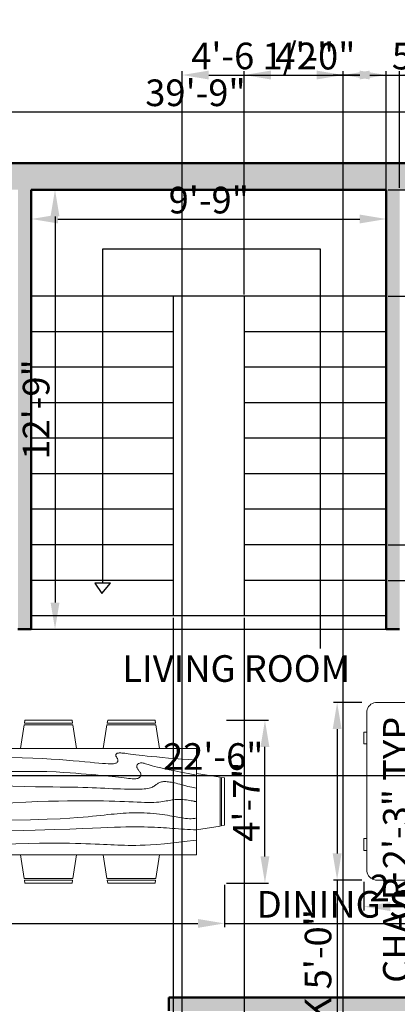
# Model space of a CAD drawing. Units: inches. Extents: x 875413 to 876020, y 447446 to 448210.
# Tile 6 of 8: x 875639 to 875767, y 447795 to 448127. Entities that reach past the tile are written whole.
import ezdxf

# ---------------------------------------------------------------- set-up
doc = ezdxf.new("R2010")
doc.units = ezdxf.units.IN
for name, color, linetype, lineweight in [('A-ANNO-DIMS', 2, 'Continuous', 13), ('A-AREA-IDEN', 7, 'Continuous', 25), ('A-FLOR-STRS', 7, 'Continuous', 25), ('A-FURN', 8, 'Continuous', 18), ('A-WALL', 7, 'Continuous', 50)]:
    doc.layers.add(name, color=color, linetype=linetype, lineweight=lineweight)
doc.layers.add('A-WALL-PATT', color=18, linetype='Continuous', lineweight=13, true_color=0x000000)
doc.styles.get("Standard").update_dxf_attribs({"font": 'arial.ttf'})
doc.dimstyles.new('ISO-25', dxfattribs={"dimtxt": 9, "dimasz": 9, "dimexe": 1.25, "dimexo": 0.625, "dimtad": 1, "dimdec": 1, "dimrnd": 9, "dimlunit": 3, "dimtxsty": 'Standard', "dimcen": 2.5, "dimadec": 0, "dimazin": 0, "dimtfac": 1, "dimtdec": 1, "dimtmove": 0, "dimatfit": 3, "dimfxl": 1, "dimarcsym": 0})

# ---------------------------------------------------------------- blocks, each defined once
blk = doc.blocks.new('*D3')
at = {"layer": 'A-ANNO-DIMS', "color": 0, "lineweight": -2, "transparency": 16777216}
for p, q in [((875643.2, 448069.39), (875643.2, 448058.87)), ((875763.2, 448069.39), (875763.2, 448058.87)), ((875652.2, 448060.12), (875754.2, 448060.12))]:
    blk.add_line(p, q, dxfattribs=at)
at = {"layer": 'A-ANNO-DIMS', "color": 0, "transparency": 16777216}
for points in [[(875652.2, 448061.62), (875652.2, 448058.62), (875643.2, 448060.12)], [(875754.2, 448061.62), (875754.2, 448058.62), (875763.2, 448060.12)]]:
    blk.add_solid(points, dxfattribs=at)
at = {"layer": 'Defpoints', "color": 0, "transparency": 16777216}
for p in [(875643.2, 448070.02), (875763.2, 448070.02), (875763.2, 448060.12)]:
    blk.add_point(p, dxfattribs=at)
at = {"layer": 'A-ANNO-DIMS', "color": 0, "transparency": 16777216, "insert": (875703.2, 448065.34), "char_height": 9, "attachment_point": 5}
blk.add_mtext('9\'-9"', dxfattribs=at)
blk = doc.blocks.new('*D4')
at = {"layer": 'A-ANNO-DIMS', "color": 0, "lineweight": -2, "transparency": 16777216}
for p, q in [((875643.83, 448070.02), (875652.48, 448070.02)), ((875651.23, 448061.02), (875651.23, 447930.52)), ((875643.83, 447921.52), (875652.48, 447921.52))]:
    blk.add_line(p, q, dxfattribs=at)
at = {"layer": 'A-ANNO-DIMS', "color": 0, "transparency": 16777216}
for points in [[(875649.73, 448061.02), (875652.73, 448061.02), (875651.23, 448070.02)], [(875649.73, 447930.52), (875652.73, 447930.52), (875651.23, 447921.52)]]:
    blk.add_solid(points, dxfattribs=at)
at = {"layer": 'Defpoints', "color": 0, "transparency": 16777216}
for p in [(875643.2, 448070.02), (875643.2, 447921.52), (875651.23, 447921.52)]:
    blk.add_point(p, dxfattribs=at)
at = {"layer": 'A-ANNO-DIMS', "color": 0, "transparency": 16777216, "insert": (875646.01, 447995.77), "char_height": 9, "attachment_point": 5, "rotation": 90}
blk.add_mtext('12\'-9"', dxfattribs=at)
blk = doc.blocks.new('*D13')
at = {"layer": 'A-ANNO-DIMS', "color": 0, "lineweight": -2, "transparency": 16777216}
for p, q in [((875571.2, 447920.89), (875571.2, 447870.86)), ((875838.2, 447920.89), (875838.2, 447870.86)), ((875580.2, 447872.11), (875829.2, 447872.11))]:
    blk.add_line(p, q, dxfattribs=at)
at = {"layer": 'A-ANNO-DIMS', "color": 0, "transparency": 16777216}
for points in [[(875580.2, 447873.61), (875580.2, 447870.61), (875571.2, 447872.11)], [(875829.2, 447873.61), (875829.2, 447870.61), (875838.2, 447872.11)]]:
    blk.add_solid(points, dxfattribs=at)
at = {"layer": 'Defpoints', "color": 0, "transparency": 16777216}
for p in [(875571.2, 447921.52), (875838.2, 447921.52), (875838.2, 447872.11)]:
    blk.add_point(p, dxfattribs=at)
at = {"layer": 'A-ANNO-DIMS', "color": 0, "transparency": 16777216, "insert": (875704.7, 447877.33), "char_height": 9, "attachment_point": 5}
blk.add_mtext('22\'-6"', dxfattribs=at)
blk = doc.blocks.new('Dining Set - 36 x 72 in.')
for p, q in [((-22, 27.5), (-22.1562, 26.50042)), ((-22, 27.5), (-6, 27.5)), ((-5.8437, 26.49966), (-6, 27.5)), ((6, 27.5), (5.8438, 26.50042)), ((6, 27.5), (22, 27.5)), ((22.1563, 26.49966), (22, 27.5)), ((-22.2343, 26.00059), (-23.4847, 17.99762)), ((-22.2304, 26), (-5.7608, 26)), ((-5.8416, 26.5), (-22.1534, 26.5)), ((-4.5152, 17.99762), (-5.7655, 25.99926)), ((5.7657, 26.00059), (4.5153, 17.99762)), ((5.7696, 26), (22.2392, 26)), ((22.1584, 26.5), (5.8466, 26.5)), ((23.4848, 17.99762), (22.2345, 25.99926)), ((36, 18), (-36, 18)), ((-36, 18), (-36, -18)), ((36, -18), (36, 18)), ((-45.5, 8), (-44.5004, 8.15617)), ((-45.5, 8), (-45.5, -8)), ((-44.5, -8.15843), (-44.5, 8.15338)), ((-44.0006, 8.23428), (-35.9976, 9.48474)), ((-44, 8.23041), (-44, -8.23915)), ((44.0006, 8.23428), (35.9976, 9.48474)), ((44, 8.23041), (44, -8.23915)), ((44.5, -8.15843), (44.5, 8.15338)), ((45.5, 8), (44.5005, 8.15617)), ((45.5, 8), (45.5, -8)), ((-44.4997, -8.15631), (-45.5, -8)), ((-35.9976, -9.48476), (-43.9993, -8.2345)), ((35.9976, -9.48476), (43.9993, -8.2345)), ((44.4997, -8.15631), (45.5, -8)), ((-36, -18), (36, -18)), ((-22.2343, -26.0006), (-23.4847, -17.99762)), ((-4.5152, -17.99762), (-5.7655, -25.99928)), ((5.7657, -26.0006), (4.5153, -17.99762)), ((23.4848, -17.99762), (22.2345, -25.99928)), ((-22.2304, -26), (-5.7608, -26)), ((-22, -27.5), (-22.1562, -26.50044)), ((-5.8416, -26.5), (-22.1534, -26.5)), ((-5.8437, -26.49967), (-6, -27.5)), ((5.7696, -26), (22.2392, -26)), ((6, -27.5), (5.8438, -26.50044)), ((22.1584, -26.5), (5.8466, -26.5)), ((22.1563, -26.49967), (22, -27.5)), ((-22, -27.5), (-6, -27.5)), ((6, -27.5), (22, -27.5))]:
    blk.add_line(p, q)
for points in [[(-36, 15), (-31.1772, 14.97754), (-26.8079, 14.91406), (-22.8538, 14.81543), (-19.276, 14.6875), (-16.0362, 14.53613), (-13.0957, 14.36718), (-10.4159, 14.18652), (-7.9583, 14), (-5.6904, 13.81315), (-3.6035, 13.63021), (-1.6954, 13.45508), (0.0365, 13.29166), (1.5945, 13.14388), (2.9811, 13.01562), (4.1988, 12.9108), (5.25, 12.83333), (6.1393, 12.78613), (6.8802, 12.76823), (7.4883, 12.77767), (7.9792, 12.8125), (8.3685, 12.87077), (8.6719, 12.95052), (8.9049, 13.0498), (9.0833, 13.16666), (9.2205, 13.29899), (9.3216, 13.44401), (9.3895, 13.59879), (9.4271, 13.76041), (9.4373, 13.92594), (9.4232, 14.09245), (9.3875, 14.257), (9.3333, 14.41666), (9.2638, 14.56917), (9.1836, 14.71484), (9.0975, 14.85465), (9.0104, 14.98958), (8.9272, 15.1206), (8.8529, 15.2487), (8.7922, 15.37483), (8.75, 15.5), (8.7305, 15.62467), (8.7344, 15.74739), (8.7617, 15.86621), (8.8125, 15.97916), (8.8867, 16.08431), (8.9844, 16.17968), (9.1055, 16.26334), (9.25, 16.33333), (9.4189, 16.38802), (9.6172, 16.42708), (9.8506, 16.45052), (10.125, 16.45833), (10.4463, 16.45052), (10.8203, 16.42708), (11.2529, 16.38802), (11.75, 16.33333), (12.3184, 16.26318), (12.9694, 16.17838), (13.7151, 16.07991), (14.5677, 15.96875), (15.5395, 15.84586), (16.6426, 15.71224), (17.8893, 15.56884), (19.2917, 15.41666), (20.859, 15.25667), (22.5879, 15.08984), (24.4721, 14.91715), (26.5052, 14.73958), (28.6809, 14.5581), (30.9929, 14.3737), (33.4347, 14.18733), (36, 14)], [(-36, 10), (-28.9766, 10.14274), (-23.1725, 10.20442), (-18.4241, 10.19775), (-14.5677, 10.13541), (-11.4399, 10.03011), (-8.877, 9.89453), (-6.7154, 9.74137), (-4.7917, 9.58333), (-2.9698, 9.43082), (-1.2246, 9.28515), (0.4415, 9.14534), (2.026, 9.01041), (3.5266, 8.87939), (4.9408, 8.7513), (6.266, 8.62516), (7.5, 8.5), (8.6411, 8.37549), (9.6914, 8.2539), (10.6538, 8.13818), (11.5312, 8.03125), (12.3267, 7.93603), (13.043, 7.85547), (13.6831, 7.79248), (14.25, 7.75), (14.7471, 7.7303), (15.1797, 7.73307), (15.5537, 7.75732), (15.875, 7.80208), (16.1494, 7.86637), (16.3828, 7.94922), (16.5811, 8.04964), (16.75, 8.16666), (16.8944, 8.29915), (17.0143, 8.44531), (17.1089, 8.60319), (17.1771, 8.77083), (17.218, 8.94629), (17.2305, 9.1276), (17.2137, 9.31282), (17.1667, 9.5), (17.0895, 9.6875), (16.987, 9.875), (16.8649, 10.0625), (16.7292, 10.25), (16.5856, 10.4375), (16.4401, 10.625), (16.2985, 10.8125), (16.1667, 11), (16.05, 11.18733), (15.9518, 11.3737), (15.8752, 11.5581), (15.8229, 11.73958), (15.798, 11.91715), (15.8034, 12.08984), (15.842, 12.25667), (15.9167, 12.41666), (16.0295, 12.56836), (16.1784, 12.70833), (16.3605, 12.83268), (16.5729, 12.9375), (16.8127, 13.01888), (17.0768, 13.07291), (17.3625, 13.0957), (17.6667, 13.08333), (17.9894, 13.03312), (18.3418, 12.94726), (18.7382, 12.82918), (19.1927, 12.68229), (19.7195, 12.51001), (20.3327, 12.31575), (21.0465, 12.10294), (21.875, 11.875), (22.8357, 11.63354), (23.959, 11.37304), (25.2786, 11.08618), (26.8282, 10.76562), (28.6414, 10.40405), (30.752, 9.99414), (33.1936, 9.52856), (36, 9)], [(-36, 5.5), (-30.7157, 5.3348), (-26.069, 5.20963), (-21.9946, 5.11767), (-18.4271, 5.05208), (-15.3009, 5.00602), (-12.5508, 4.97265), (-10.1112, 4.94515), (-7.9167, 4.91666), (-5.909, 4.88167), (-4.0586, 4.83984), (-2.3429, 4.79215), (-0.7396, 4.73958), (0.7739, 4.6831), (2.22, 4.6237), (3.6213, 4.56233), (5, 4.5), (6.373, 4.43782), (7.7344, 4.3776), (9.0723, 4.32129), (10.375, 4.27083), (11.6309, 4.22819), (12.8281, 4.19531), (13.9551, 4.17415), (15, 4.16666), (15.954, 4.17448), (16.819, 4.19791), (17.6001, 4.23698), (18.3021, 4.29166), (18.9299, 4.36198), (19.4883, 4.44791), (19.9823, 4.54948), (20.4167, 4.66666), (20.7969, 4.79899), (21.1302, 4.94401), (21.4245, 5.09879), (21.6875, 5.26041), (21.9271, 5.42594), (22.1511, 5.59245), (22.3672, 5.757), (22.5834, 5.91666), (22.8065, 6.06868), (23.0404, 6.21093), (23.2879, 6.34147), (23.5521, 6.45833), (23.8358, 6.55957), (24.142, 6.64323), (24.4735, 6.70735), (24.8334, 6.75), (25.2235, 6.76969), (25.642, 6.76692), (26.0858, 6.74267), (26.5521, 6.69791), (27.0379, 6.63362), (27.5404, 6.55078), (28.0565, 6.45036), (28.5834, 6.33333), (29.1242, 6.19987), (29.7071, 6.04687), (30.3661, 5.87044), (31.1354, 5.66666), (32.0493, 5.43164), (33.142, 5.16146), (34.4475, 4.85221), (36, 4.5)], [(-36, -1), (-30.7915, -0.6591), (-26.0195, -0.38216), (-21.6519, -0.16284), (-17.6563, 0.00521), (-14.0005, 0.12833), (-10.6523, 0.21289), (-7.5796, 0.26522), (-4.75, 0.29166), (-2.134, 0.29793), (0.2878, 0.28711), (2.5317, 0.26163), (4.6146, 0.22396), (6.5529, 0.17651), (8.3633, 0.12174), (10.0623, 0.06209), (11.6667, 0), (13.1899, -0.06201), (14.6341, -0.1211), (15.9982, -0.17432), (17.2813, -0.21875), (18.4823, -0.25147), (19.6003, -0.26953), (20.6343, -0.27002), (21.5834, -0.25), (22.4481, -0.20768), (23.2357, -0.14584), (23.9549, -0.06836), (24.6146, 0.02083), (25.2235, 0.11784), (25.7904, 0.21875), (26.3241, 0.31966), (26.8334, 0.41666), (27.3265, 0.50618), (27.8099, 0.58593), (28.2894, 0.65397), (28.7709, 0.70833), (29.2601, 0.74707), (29.763, 0.76823), (30.2855, 0.76985), (30.8334, 0.75), (31.4088, 0.70784), (31.9994, 0.64713), (32.589, 0.57275), (33.1615, 0.48958), (33.7008, 0.4025), (34.1908, 0.3164), (34.6153, 0.23616), (34.9584, 0.16666), (35.2099, 0.11165), (35.3848, 0.07031), (35.504, 0.04069), (35.5886, 0.02083), (35.6594, 0.00879), (35.7377, 0.0026), (35.8442, 0.00032), (36, 0)], [(-36, -6.5), (-27.1843, -6.31267), (-20.084, -6.1263), (-14.469, -5.9419), (-10.1094, -5.76042), (-6.7752, -5.58285), (-4.2363, -5.41016), (-2.2629, -5.24333), (-0.625, -5.08334), (0.8708, -4.93099), (2.2715, -4.78646), (3.5872, -4.64974), (4.8281, -4.52084), (6.0046, -4.39974), (7.127, -4.28646), (8.2053, -4.18099), (9.25, -4.08334), (10.2705, -3.99382), (11.2734, -3.91407), (12.2647, -3.84603), (13.25, -3.79167), (14.2354, -3.75293), (15.2266, -3.73177), (16.2295, -3.73015), (17.25, -3.75), (18.2912, -3.79248), (19.3451, -3.85547), (20.4009, -3.93604), (21.4479, -4.03125), (22.4754, -4.13819), (23.4727, -4.25391), (24.4289, -4.37549), (25.3334, -4.5), (26.1785, -4.62492), (26.9694, -4.74935), (27.7145, -4.87281), (28.4219, -4.99479), (29.1, -5.11483), (29.7572, -5.23242), (30.4016, -5.34709), (31.0417, -5.45834), (31.6837, -5.56437), (32.3262, -5.65821), (32.9658, -5.73153), (33.599, -5.77604), (34.2224, -5.78345), (34.8327, -5.74545), (35.4264, -5.65373), (36, -5.5)], [(-36, -10), (-26.4022, -9.81299), (-18.4675, -9.62891), (-11.9839, -9.45069), (-6.7396, -9.28125), (-2.5226, -9.12354), (0.8789, -8.98047), (3.6769, -8.85498), (6.0833, -8.75), (8.2767, -8.66765), (10.3021, -8.60677), (12.1712, -8.56543), (13.8958, -8.54167), (15.4876, -8.53353), (16.9583, -8.53907), (18.3197, -8.55632), (19.5834, -8.58334), (20.7616, -8.61841), (21.8685, -8.66081), (22.9188, -8.71004), (23.9271, -8.76563), (24.9081, -8.82707), (25.8763, -8.89388), (26.8465, -8.96558), (27.8334, -9.04167), (28.8474, -9.12118), (29.8828, -9.20117), (30.93, -9.27824), (31.9792, -9.34896), (33.0205, -9.40991), (34.0443, -9.45768), (35.0407, -9.48885), (36, -9.5)], [(-36, -14.5), (-30.0881, -14.33513), (-25.0332, -14.21224), (-20.7312, -14.12647), (-17.0781, -14.07292), (-13.97, -14.04671), (-11.3027, -14.04297), (-8.9724, -14.05681), (-6.875, -14.08334), (-4.9224, -14.11833), (-3.0905, -14.16016), (-1.3709, -14.20785), (0.2448, -14.26042), (1.7647, -14.3169), (3.1973, -14.3763), (4.5507, -14.43767), (5.8333, -14.5), (7.0554, -14.5621), (8.235, -14.62175), (9.3922, -14.67652), (10.5469, -14.72396), (11.7192, -14.76164), (12.929, -14.78711), (14.1965, -14.79794), (15.5417, -14.79167), (16.9933, -14.76424), (18.6152, -14.70508), (20.4804, -14.60197), (22.6615, -14.44271), (25.2312, -14.21509), (28.2624, -13.9069), (31.8277, -13.50594), (36, -13)]]:
    blk.add_lwpolyline(points)
blk = doc.blocks.new('Desk - 30 x 60 in.')
for p, q in [((-26.999995, 0), (26.999995, 0)), ((-29.999995, -27), (-29.999995, -3)), ((29.999995, -3), (29.999995, -27)), ((26.999995, -30), (-26.999995, -30)), ((-20.000005, -30), (-20.000005, -31)), ((-20.000005, -31), (-16.000005, -31)), ((-16.000005, -31), (-16.000005, -30)), ((15.999995, -31), (15.999995, -30)), ((19.999995, -31), (15.999995, -31)), ((19.999995, -30), (19.999995, -31))]:
    blk.add_line(p, q)
for centre, start, end in [((-26.499995, -3.5), 98.1301, 171.8699), ((26.499995, -3.5), 8.130102, 81.8699), ((-26.499995, -26.5), 188.1301, 261.8699), ((26.499995, -26.5), 278.1301, 351.8699)]:
    blk.add_arc(centre, 3.535534, start, end)
blk = doc.blocks.new('*D37')
at = {"layer": 'A-ANNO-DIMS', "color": 0, "lineweight": -2, "transparency": 16777216}
for p, q in [((875461.7, 448079.64), (875461.7, 448097.63)), ((875470.7, 448096.38), (875926.7, 448096.38)), ((875935.7, 448079.64), (875935.7, 448097.63))]:
    blk.add_line(p, q, dxfattribs=at)
at = {"layer": 'A-ANNO-DIMS', "color": 0, "transparency": 16777216}
for points in [[(875470.7, 448097.88), (875470.7, 448094.88), (875461.7, 448096.38)], [(875926.7, 448097.88), (875926.7, 448094.88), (875935.7, 448096.38)]]:
    blk.add_solid(points, dxfattribs=at)
at = {"layer": 'Defpoints', "color": 0, "transparency": 16777216}
for p in [(875935.7, 448096.38), (875461.7, 448079.02), (875935.7, 448079.02)]:
    blk.add_point(p, dxfattribs=at)
at = {"layer": 'A-ANNO-DIMS', "color": 0, "transparency": 16777216, "insert": (875698.7, 448101.6), "char_height": 9, "attachment_point": 5}
blk.add_mtext('39\'-9"', dxfattribs=at)
blk = doc.blocks.new('*D53')
at = {"layer": 'A-ANNO-DIMS', "color": 0, "lineweight": -2, "transparency": 16777216}
for p, q in [((875617.53, 447835.12), (875617.53, 447820.85)), ((875708.53, 447835.12), (875708.53, 447820.85)), ((875626.53, 447822.1), (875699.53, 447822.1)), ((875708.53, 447822.1), (875817.7, 447822.1))]:
    blk.add_line(p, q, dxfattribs=at)
at = {"layer": 'A-ANNO-DIMS', "color": 0, "transparency": 16777216}
for points in [[(875626.53, 447823.6), (875626.53, 447820.6), (875617.53, 447822.1)], [(875699.53, 447823.6), (875699.53, 447820.6), (875708.53, 447822.1)]]:
    blk.add_solid(points, dxfattribs=at)
at = {"layer": 'Defpoints', "color": 0, "transparency": 16777216}
for p in [(875617.53, 447835.75), (875708.53, 447835.75), (875708.53, 447822.1)]:
    blk.add_point(p, dxfattribs=at)
at = {"layer": 'A-ANNO-DIMS', "color": 0, "transparency": 16777216, "insert": (875767.62, 447827.38), "char_height": 9, "attachment_point": 5}
blk.add_mtext('DINING SET 7\'-7"', dxfattribs=at)
blk = doc.blocks.new('*D54')
at = {"layer": 'A-ANNO-DIMS', "color": 0, "lineweight": -2, "transparency": 16777216}
for p, q in [((875709.16, 447890.75), (875723.43, 447890.75)), ((875722.18, 447844.75), (875722.18, 447881.75)), ((875709.16, 447835.75), (875723.43, 447835.75))]:
    blk.add_line(p, q, dxfattribs=at)
at = {"layer": 'A-ANNO-DIMS', "color": 0, "transparency": 16777216}
for points in [[(875720.68, 447881.75), (875723.68, 447881.75), (875722.18, 447890.75)], [(875720.68, 447844.75), (875723.68, 447844.75), (875722.18, 447835.75)]]:
    blk.add_solid(points, dxfattribs=at)
at = {"layer": 'Defpoints', "color": 0, "transparency": 16777216}
for p in [(875708.53, 447890.75), (875722.18, 447890.75), (875708.53, 447835.75)]:
    blk.add_point(p, dxfattribs=at)
at = {"layer": 'A-ANNO-DIMS', "color": 0, "transparency": 16777216, "insert": (875717.06, 447863.25), "char_height": 9, "attachment_point": 5, "rotation": 90}
blk.add_mtext('4\'-7"', dxfattribs=at)
blk = doc.blocks.new('*D57')
at = {"layer": 'A-ANNO-DIMS', "color": 0, "lineweight": -2, "transparency": 16777216}
for p, q in [((875773.04, 447790.36), (875773.04, 447897.98)), ((875776.46, 447790.36), (875771.79, 447790.36)), ((875773.04, 447772.36), (875773.04, 447781.36)), ((875776.46, 447763.36), (875771.79, 447763.36))]:
    blk.add_line(p, q, dxfattribs=at)
at = {"layer": 'A-ANNO-DIMS', "color": 0, "transparency": 16777216}
for points in [[(875771.54, 447781.36), (875774.54, 447781.36), (875773.04, 447790.36)], [(875771.54, 447772.36), (875774.54, 447772.36), (875773.04, 447763.36)]]:
    blk.add_solid(points, dxfattribs=at)
at = {"layer": 'Defpoints', "color": 0, "transparency": 16777216}
for p in [(875773.04, 447790.36), (875777.09, 447790.36), (875777.09, 447763.36)]:
    blk.add_point(p, dxfattribs=at)
at = {"layer": 'A-ANNO-DIMS', "color": 0, "transparency": 16777216, "insert": (875767.76, 447848.67), "char_height": 9, "attachment_point": 5, "rotation": 90}
blk.add_mtext('CHAIR 2\'-3" TYP.', dxfattribs=at)
blk = doc.blocks.new('*D61')
at = {"layer": 'A-ANNO-DIMS', "color": 0, "lineweight": -2, "transparency": 16777216}
for p, q in [((875754.96, 447896.77), (875745.33, 447896.77)), ((875746.58, 447887.77), (875746.58, 447845.77)), ((875754.96, 447836.77), (875745.33, 447836.77)), ((875746.58, 447836.77), (875746.58, 447765.31))]:
    blk.add_line(p, q, dxfattribs=at)
at = {"layer": 'A-ANNO-DIMS', "color": 0, "transparency": 16777216}
for points in [[(875745.08, 447887.77), (875748.08, 447887.77), (875746.58, 447896.77)], [(875745.08, 447845.77), (875748.08, 447845.77), (875746.58, 447836.77)]]:
    blk.add_solid(points, dxfattribs=at)
at = {"layer": 'Defpoints', "color": 0, "transparency": 16777216}
for p in [(875755.58, 447896.77), (875746.58, 447836.77), (875755.58, 447836.77)]:
    blk.add_point(p, dxfattribs=at)
at = {"layer": 'A-ANNO-DIMS', "color": 0, "transparency": 16777216, "insert": (875741.3, 447796.54), "char_height": 9, "attachment_point": 5, "rotation": 90}
blk.add_mtext('DESK 5\'-0"', dxfattribs=at)
blk = doc.blocks.new('*D62')
at = {"layer": 'A-ANNO-DIMS', "color": 0, "lineweight": -2, "transparency": 16777216}
for p, q in [((875755.58, 447836.14), (875755.58, 447826.52)), ((875786.58, 447836.14), (875786.58, 447826.52)), ((875764.58, 447827.77), (875777.58, 447827.77))]:
    blk.add_line(p, q, dxfattribs=at)
at = {"layer": 'A-ANNO-DIMS', "color": 0, "transparency": 16777216}
for points in [[(875764.58, 447829.27), (875764.58, 447826.27), (875755.58, 447827.77)], [(875777.58, 447829.27), (875777.58, 447826.27), (875786.58, 447827.77)]]:
    blk.add_solid(points, dxfattribs=at)
at = {"layer": 'Defpoints', "color": 0, "transparency": 16777216}
for p in [(875755.58, 447836.77), (875786.58, 447836.77), (875786.58, 447827.77)]:
    blk.add_point(p, dxfattribs=at)
at = {"layer": 'A-ANNO-DIMS', "color": 0, "transparency": 16777216, "insert": (875771.08, 447832.91), "char_height": 9, "attachment_point": 5}
blk.add_mtext('2\'-7"', dxfattribs=at)
blk = doc.blocks.new('*D77')
at = {"layer": 'A-ANNO-DIMS', "color": 0, "lineweight": -2, "transparency": 16777216}
for p, q in [((875715.2, 448034.64), (875715.2, 448110.02)), ((875763.2, 448034.64), (875763.2, 448110.02)), ((875724.2, 448108.77), (875754.2, 448108.77))]:
    blk.add_line(p, q, dxfattribs=at)
at = {"layer": 'A-ANNO-DIMS', "color": 0, "transparency": 16777216}
for points in [[(875724.2, 448110.27), (875724.2, 448107.27), (875715.2, 448108.77)], [(875754.2, 448110.27), (875754.2, 448107.27), (875763.2, 448108.77)]]:
    blk.add_solid(points, dxfattribs=at)
at = {"layer": 'Defpoints', "color": 0, "transparency": 16777216}
for p in [(875763.2, 448108.77), (875715.2, 448034.02), (875763.2, 448034.02)]:
    blk.add_point(p, dxfattribs=at)
at = {"layer": 'A-ANNO-DIMS', "color": 0, "transparency": 16777216, "insert": (875739.2, 448113.99), "char_height": 9, "attachment_point": 5}
blk.add_mtext('4\'-0"', dxfattribs=at)
blk = doc.blocks.new('*D78')
at = {"layer": 'A-ANNO-DIMS', "color": 0, "lineweight": -2, "transparency": 16777216}
for p, q in [((875965.45, 447959.02), (875965.45, 447992.34)), ((875763.83, 447950.02), (875966.7, 447950.02)), ((875965.45, 447938.02), (875965.45, 447950.02)), ((875763.83, 447938.02), (875966.7, 447938.02)), ((875965.45, 447929.02), (875965.45, 447920.02))]:
    blk.add_line(p, q, dxfattribs=at)
at = {"layer": 'A-ANNO-DIMS', "color": 0, "transparency": 16777216}
for points in [[(875963.95, 447959.02), (875966.95, 447959.02), (875965.45, 447950.02)], [(875963.95, 447929.02), (875966.95, 447929.02), (875965.45, 447938.02)]]:
    blk.add_solid(points, dxfattribs=at)
at = {"layer": 'Defpoints', "color": 0, "transparency": 16777216}
for p in [(875763.2, 447950.02), (875965.45, 447950.02), (875763.2, 447938.02)]:
    blk.add_point(p, dxfattribs=at)
at = {"layer": 'A-ANNO-DIMS', "color": 0, "transparency": 16777216, "insert": (875960.23, 447980.18), "char_height": 9, "attachment_point": 5, "rotation": 90}
blk.add_mtext('1\'-0"', dxfattribs=at)
blk = doc.blocks.new('*D79')
at = {"layer": 'A-ANNO-DIMS', "color": 0, "lineweight": -2, "transparency": 16777216}
for p, q in [((875694.2, 447673.14), (875694.2, 448110.02)), ((875748.63, 447673.14), (875748.63, 448110.02)), ((875703.2, 448108.77), (875739.63, 448108.77))]:
    blk.add_line(p, q, dxfattribs=at)
at = {"layer": 'A-ANNO-DIMS', "color": 0, "transparency": 16777216}
for points in [[(875703.2, 448110.27), (875703.2, 448107.27), (875694.2, 448108.77)], [(875739.63, 448110.27), (875739.63, 448107.27), (875748.63, 448108.77)]]:
    blk.add_solid(points, dxfattribs=at)
at = {"layer": 'Defpoints', "color": 0, "transparency": 16777216}
for p in [(875748.63, 448108.77), (875694.2, 447672.52), (875748.63, 447672.52)]:
    blk.add_point(p, dxfattribs=at)
at = {"layer": 'A-ANNO-DIMS', "color": 0, "transparency": 16777216, "insert": (875721.42, 448114.05), "char_height": 9, "attachment_point": 5}
blk.add_mtext('4\'-6 1/2"', dxfattribs=at)
blk = doc.blocks.new('*D80')
at = {"layer": 'A-ANNO-DIMS', "color": 0, "lineweight": -2, "transparency": 16777216}
for p, q in [((875748.63, 447673.14), (875748.63, 448110.02)), ((875808.63, 447673.14), (875808.63, 448110.02)), ((875757.63, 448108.77), (875799.63, 448108.77))]:
    blk.add_line(p, q, dxfattribs=at)
at = {"layer": 'A-ANNO-DIMS', "color": 0, "transparency": 16777216}
for points in [[(875757.63, 448110.27), (875757.63, 448107.27), (875748.63, 448108.77)], [(875799.63, 448110.27), (875799.63, 448107.27), (875808.63, 448108.77)]]:
    blk.add_solid(points, dxfattribs=at)
at = {"layer": 'Defpoints', "color": 0, "transparency": 16777216}
for p in [(875808.63, 448108.77), (875748.63, 447672.52), (875808.63, 447672.52)]:
    blk.add_point(p, dxfattribs=at)
at = {"layer": 'A-ANNO-DIMS', "color": 0, "transparency": 16777216, "insert": (875778.63, 448113.99), "char_height": 9, "attachment_point": 5}
blk.add_mtext('5\'-0"', dxfattribs=at)
blk = doc.blocks.new('*D81')
at = {"layer": 'A-ANNO-DIMS', "color": 0, "lineweight": -2, "transparency": 16777216}
for p, q in [((875763.2, 448070.64), (875763.2, 448110.02)), ((875767.7, 448070.64), (875767.7, 448110.02)), ((875754.2, 448108.77), (875745.2, 448108.77)), ((875763.2, 448108.77), (875767.7, 448108.77)), ((875776.7, 448108.77), (875831.85, 448108.77))]:
    blk.add_line(p, q, dxfattribs=at)
at = {"layer": 'A-ANNO-DIMS', "color": 0, "transparency": 16777216}
for points in [[(875754.2, 448110.27), (875754.2, 448107.27), (875763.2, 448108.77)], [(875776.7, 448110.27), (875776.7, 448107.27), (875767.7, 448108.77)]]:
    blk.add_solid(points, dxfattribs=at)
at = {"layer": 'Defpoints', "color": 0, "transparency": 16777216}
for p in [(875767.7, 448108.77), (875763.2, 448070.02), (875767.7, 448070.02)]:
    blk.add_point(p, dxfattribs=at)
at = {"layer": 'A-ANNO-DIMS', "color": 0, "transparency": 16777216, "insert": (875808.78, 448114.05), "char_height": 9, "attachment_point": 5}
blk.add_mtext('0\'-4 1/2"', dxfattribs=at)
blk = doc.blocks.new('*D86')
at = {"layer": 'A-ANNO-DIMS', "color": 0, "lineweight": -2, "transparency": 16777216}
for p, q in [((875691.2, 447925.39), (875691.2, 447514.02)), ((875715.2, 447925.39), (875715.2, 447514.02)), ((875700.2, 447515.27), (875706.2, 447515.27)), ((875715.2, 447515.27), (875749.53, 447515.27))]:
    blk.add_line(p, q, dxfattribs=at)
at = {"layer": 'A-ANNO-DIMS', "color": 0, "transparency": 16777216}
for points in [[(875700.2, 447516.77), (875700.2, 447513.77), (875691.2, 447515.27)], [(875706.2, 447516.77), (875706.2, 447513.77), (875715.2, 447515.27)]]:
    blk.add_solid(points, dxfattribs=at)
at = {"layer": 'Defpoints', "color": 0, "transparency": 16777216}
for p in [(875691.2, 447926.02), (875715.2, 447926.02), (875715.2, 447515.27)]:
    blk.add_point(p, dxfattribs=at)
at = {"layer": 'A-ANNO-DIMS', "color": 0, "transparency": 16777216, "insert": (875736.87, 447520.49), "char_height": 9, "attachment_point": 5}
blk.add_mtext('2\'-0"', dxfattribs=at)
blk = doc.blocks.new('*D87')
at = {"layer": 'A-ANNO-DIMS', "color": 0, "lineweight": -2, "transparency": 16777216}
for p, q in [((875763.83, 448070.02), (875966.7, 448070.02)), ((875965.45, 448043.02), (875965.45, 448061.02)), ((875763.83, 448034.02), (875966.7, 448034.02))]:
    blk.add_line(p, q, dxfattribs=at)
at = {"layer": 'A-ANNO-DIMS', "color": 0, "transparency": 16777216}
for points in [[(875963.95, 448061.02), (875966.95, 448061.02), (875965.45, 448070.02)], [(875963.95, 448043.02), (875966.95, 448043.02), (875965.45, 448034.02)]]:
    blk.add_solid(points, dxfattribs=at)
at = {"layer": 'Defpoints', "color": 0, "transparency": 16777216}
for p in [(875763.2, 448070.02), (875965.45, 448070.02), (875763.2, 448034.02)]:
    blk.add_point(p, dxfattribs=at)
at = {"layer": 'A-ANNO-DIMS', "color": 0, "transparency": 16777216, "insert": (875960.23, 448052.02), "char_height": 9, "attachment_point": 5, "rotation": 90}
blk.add_mtext('3\'-0"', dxfattribs=at)

msp = doc.modelspace()

# ---------------------------------------------------------------- hatches: boundary and pattern name
at = {"layer": 'A-WALL-PATT'}
h = msp.add_hatch(color=256, dxfattribs=at)
h.dxf.hatch_style = 1
h.paths.add_polyline_path([(875470.7, 447985.13), (875461.7, 447985.13), (875461.7, 447865.29), (875470.7, 447865.29), (875470.7, 447881.02), (875566.7, 447881.02), (875566.7, 447797.02), (875571.2, 447797.02), (875571.2, 447885.52), (875571.2, 447921.52), (875603.29, 447921.52), (875603.29, 447926.02), (875501.27, 447926.02), (875501.27, 447921.52), (875566.7, 447921.52), (875566.7, 447885.52), (875470.7, 447885.52), (875470.7, 447921.52), (875470.7, 447926.02)])
h.paths.add_polyline_path([(875470.7, 448070.02), (875518.96, 448070.02), (875518.96, 448079.02), (875461.7, 448079.02), (875461.7, 448045.13), (875470.7, 448045.13)])
h.paths.add_polyline_path([(875819.9, 448079.02), (875578.96, 448079.02), (875578.96, 448070.02), (875638.7, 448070.02), (875638.7, 447921.52), (875643.2, 447921.52), (875643.2, 448070.02), (875763.2, 448070.02), (875763.2, 447921.52), (875767.7, 447921.52), (875767.7, 448070.02), (875819.9, 448070.02)])
h.paths.add_polyline_path([(875935.7, 447978.92), (875926.7, 447978.92), (875926.7, 447926.02), (875926.7, 447921.52), (875926.7, 447885.52), (875842.7, 447885.52), (875842.7, 447921.52), (875899.7, 447921.52), (875899.7, 447926.02), (875805.34, 447926.02), (875805.34, 447921.52), (875838.2, 447921.52), (875838.2, 447885.52), (875838.2, 447797.02), (875689.7, 447797.02), (875689.7, 447792.52), (875842.7, 447792.52), (875842.7, 447881.02), (875926.7, 447881.02), (875926.7, 447857.16), (875935.7, 447857.16)])
h.paths.add_polyline_path([(875935.7, 448079.02), (875879.9, 448079.02), (875879.9, 448070.02), (875926.7, 448070.02), (875926.7, 448038.92), (875935.7, 448038.92)])
h.paths.add_polyline_path([(875935.7, 447833.16), (875926.7, 447833.16), (875926.7, 447797.02), (875842.7, 447797.02), (875842.7, 447792.52), (875926.7, 447792.52), (875926.7, 447756.52), (875935.7, 447756.52)])
h.paths.add_polyline_path([(875935.7, 447732.52), (875926.7, 447732.52), (875926.7, 447692.75, -0.007222), (875926.81, 447692.41, -0.08192), (875927.45, 447687.6, -0.071798), (875926.7, 447683.4), (875926.7, 447672.52), (875808.63, 447672.52), (875808.63, 447668.02), (875926.7, 447668.02), (875926.7, 447663.19), (875935.7, 447663.19)])
h.paths.add_polyline_path([(875842.7, 447792.52), (875838.2, 447792.52), (875838.2, 447704.02), (875842.7, 447704.02)])
h.paths.add_polyline_path([(875470.7, 447792.52), (875619.2, 447792.52), (875619.2, 447797.02), (875470.7, 447797.02), (875470.7, 447841.29), (875461.7, 447841.29), (875461.7, 447764.71), (875470.7, 447764.71)])
h.paths.add_polyline_path([(875619.2, 447760.51), (875616.95, 447760.51, -0.018388), (875614.7, 447760.37), (875614.7, 447672.52), (875470.7, 447672.52), (875470.7, 447704.71), (875461.7, 447704.71), (875461.7, 447640.7), (875470.7, 447640.7), (875470.7, 447668.02), (875619.2, 447668.02)])
h.paths.add_polyline_path([(875511.12, 447554.02), (875470.7, 447554.02), (875470.7, 447580.7), (875461.7, 447580.7), (875461.7, 447545.02), (875511.12, 447545.02)])
h.paths.add_polyline_path([(875656.47, 447554.02), (875620.05, 447554.02, -0.057036), (875616.67, 447553.74, -0.040891), (875614.26, 447554.02), (875571.12, 447554.02), (875571.12, 447545.02), (875656.47, 447545.02)])
h.paths.add_polyline_path([(875643.2, 447613.27), (875685.21, 447613.27), (875685.21, 447617.77), (875685.21, 447623.8), (875680.71, 447623.8), (875680.71, 447617.77), (875618.23, 447617.77), (875618.23, 447623.8), (875613.73, 447623.8), (875613.73, 447617.77), (875613.73, 447613.27), (875638.7, 447613.27), (875638.7, 447554.02), (875643.2, 447554.02)])
h.paths.add_polyline_path([(875694.2, 447760.28), (875689.7, 447760.28), (875689.7, 447668.02), (875748.63, 447668.02), (875748.63, 447672.52), (875694.2, 447672.52)])

# ---------------------------------------------------------------- linework, layer by layer
at = {"layer": 'A-FLOR-STRS'}
for p, q in [((875740.91, 448049.94), (875667.24, 448049.94)), ((875667.24, 448049.94), (875667.24, 447937.09)), ((875740.91, 447914.96), (875740.91, 448049.94)), ((875763.2, 448034.02), (875643.2, 448034.02)), ((875691.2, 448034.02), (875691.2, 447926.02)), ((875715.2, 448034.02), (875715.2, 447926.02)), ((875691.2, 448022.02), (875643.2, 448022.02)), ((875763.2, 448022.02), (875715.2, 448022.02)), ((875691.2, 448010.02), (875643.2, 448010.02)), ((875763.2, 448010.02), (875715.2, 448010.02)), ((875691.2, 447998.02), (875643.2, 447998.02)), ((875763.2, 447998.02), (875715.2, 447998.02)), ((875691.2, 447986.02), (875643.2, 447986.02)), ((875763.2, 447986.02), (875715.2, 447986.02)), ((875691.2, 447974.02), (875643.2, 447974.02)), ((875763.2, 447974.02), (875715.2, 447974.02)), ((875691.2, 447962.02), (875643.2, 447962.02)), ((875763.2, 447962.02), (875715.2, 447962.02)), ((875691.2, 447950.02), (875643.2, 447950.02)), ((875763.2, 447950.02), (875715.2, 447950.02)), ((875691.2, 447938.02), (875643.2, 447938.02)), ((875667.24, 447937.09), (875664.74, 447937.09)), ((875664.74, 447937.09), (875667.03, 447933.62)), ((875667.03, 447933.62), (875669.99, 447937.09)), ((875669.99, 447937.09), (875667.24, 447937.09)), ((875763.2, 447938.02), (875715.2, 447938.02)), ((875763.2, 447926.02), (875643.2, 447926.02)), ((875643.2, 447921.52), (875763.2, 447921.52))]:
    msp.add_line(p, q, dxfattribs=at)
at = {"layer": 'A-WALL'}
for p, q in [((875935.7, 448079.02), (875461.7, 448079.02)), ((875643.2, 448070.02), (875643.2, 447921.52)), ((875763.2, 448070.02), (875643.2, 448070.02)), ((875763.2, 448070.02), (875763.2, 447921.52)), ((875638.7, 447921.52), (875643.2, 447921.52)), ((875763.2, 447921.52), (875767.7, 447921.52)), ((875838.2, 447797.02), (875689.7, 447797.02)), ((875689.7, 447792.52), (875689.7, 447797.02))]:
    msp.add_line(p, q, dxfattribs=at)

# ---------------------------------------------------------------- block references
at = {"layer": 'A-FURN', "rotation": 270}
msp.add_blockref('Desk - 30 x 60 in.', (875786.58, 447866.77), dxfattribs=at)
at = {"layer": 'A-FURN'}
msp.add_blockref('Dining Set - 36 x 72 in.', (875663.03, 447863.25), dxfattribs=at)

# ---------------------------------------------------------------- texts
at = {"layer": 'A-AREA-IDEN', "insert": (875673.99, 447912.73), "char_height": 9, "attachment_point": 1}
msp.add_mtext_dynamic_manual_height_columns('LIVING ROOM', width=100.7812, gutter_width=12.5, heights=[0], dxfattribs=at)

# ---------------------------------------------------------------- dimensions: what is measured, and where the dimension line sits
at = {"layer": 'A-ANNO-DIMS'}
for base, p1, p2, override, picture, middle in [((875748.63, 448108.77), (875694.2, 447672.52), (875748.63, 447672.52), {"dimdec": 1, "dimlfac": 1, "dimrnd": 0, "dimzin": 1, "dimdsep": 46, "dimlunit": 4, "dimfrac": 2}, '*D79', (875721.42, 448114.05)), ((875767.7, 448108.77), (875763.2, 448070.02), (875767.7, 448070.02), {"dimdec": 1, "dimlfac": 1, "dimrnd": 0, "dimzin": 1, "dimdsep": 46, "dimlunit": 4, "dimfrac": 2}, '*D81', (875808.78, 448114.05)), ((875763.2, 448108.77), (875715.2, 448034.02), (875763.2, 448034.02), {"dimdec": 1, "dimlfac": 1, "dimrnd": 0, "dimzin": 1, "dimdsep": 46, "dimlunit": 4, "dimfrac": 2}, '*D77', (875739.2, 448113.99)), ((875808.63, 448108.77), (875748.63, 447672.52), (875808.63, 447672.52), {"dimdec": 1, "dimlfac": 1, "dimrnd": 0, "dimzin": 1, "dimdsep": 46, "dimlunit": 4, "dimfrac": 2}, '*D80', (875778.63, 448113.99)), ((875935.7, 448096.38), (875461.7, 448079.02), (875935.7, 448079.02), {"dimclrd": 0, "dimclre": 0, "dimclrt": 0}, '*D37', (875698.7, 448101.6)), ((875763.2, 448060.12), (875643.2, 448070.02), (875763.2, 448070.02), {"dimclrd": 0, "dimclre": 0, "dimclrt": 0}, '*D3', (875703.2, 448065.34)), ((875715.2, 447515.27), (875691.2, 447926.02), (875715.2, 447926.02), {"dimdec": 1, "dimlfac": 1, "dimrnd": 0, "dimzin": 1, "dimdsep": 46, "dimlunit": 4, "dimfrac": 2}, '*D86', (875736.87, 447520.49)), ((875838.2, 447872.11), (875571.2, 447921.52), (875838.2, 447921.52), {"dimclrd": 0, "dimclre": 0, "dimclrt": 0}, '*D13', (875704.7, 447877.33)), ((875786.58, 447827.77), (875755.58, 447836.77), (875786.58, 447836.77), {"dimdec": 1, "dimlfac": 1, "dimrnd": 0, "dimzin": 1, "dimdsep": 46, "dimlunit": 4, "dimfrac": 2}, '*D62', (875771.08, 447832.91))]:
    dim = msp.add_linear_dim(base=base, p1=p1, p2=p2, dimstyle='ISO-25', override=override, dxfattribs=at)
    dim.commit()
    dim.dimension.update_dxf_attribs({"geometry": picture, "text_midpoint": middle})
for base, p1, p2, override, picture, middle in [((875651.23, 447921.52), (875643.2, 448070.02), (875643.2, 447921.52), {"dimclrd": 0, "dimclre": 0, "dimclrt": 0}, '*D4', (875646.01, 447995.77)), ((875965.45, 448070.02), (875763.2, 448034.02), (875763.2, 448070.02), {"dimdec": 1, "dimlfac": 1, "dimrnd": 0, "dimzin": 1, "dimdsep": 46, "dimlunit": 4, "dimfrac": 2}, '*D87', (875960.23, 448052.02)), ((875965.45, 447950.02), (875763.2, 447938.02), (875763.2, 447950.02), {"dimdec": 1, "dimlfac": 1, "dimrnd": 0, "dimzin": 1, "dimdsep": 46, "dimlunit": 4, "dimfrac": 2}, '*D78', (875960.23, 447980.18)), ((875722.18, 447890.75), (875708.53, 447835.75), (875708.53, 447890.75), {"dimdec": 1, "dimlfac": 1, "dimrnd": 0, "dimzin": 1, "dimdsep": 46, "dimlunit": 4, "dimfrac": 2}, '*D54', (875717.06, 447863.25))]:
    dim = msp.add_linear_dim(base=base, p1=p1, p2=p2, angle=90, dimstyle='ISO-25', override=override, dxfattribs=at)
    dim.commit()
    dim.dimension.update_dxf_attribs({"geometry": picture, "text_midpoint": middle})
for base, p1, p2, angle, text, picture, middle in [((875746.58, 447836.77), (875755.58, 447896.77), (875755.58, 447836.77), 270, 'DESK <>', '*D61', (875741.3, 447796.54)), ((875773.04, 447790.36), (875777.09, 447763.36), (875777.09, 447790.36), 90, 'CHAIR <> TYP.', '*D57', (875767.76, 447848.67))]:
    dim = msp.add_linear_dim(base=base, p1=p1, p2=p2, angle=angle, text=text, dimstyle='ISO-25', override={"dimdec": 1, "dimlfac": 1, "dimrnd": 0, "dimzin": 1, "dimdsep": 46, "dimlunit": 4, "dimfrac": 2}, dxfattribs=at)
    dim.commit()
    dim.dimension.update_dxf_attribs({"geometry": picture, "text_midpoint": middle})
dim = msp.add_linear_dim(base=(875708.53, 447822.1), p1=(875617.53, 447835.75), p2=(875708.53, 447835.75), text='DINING SET <>', dimstyle='ISO-25', override={"dimdec": 1, "dimlfac": 1, "dimrnd": 0, "dimzin": 1, "dimdsep": 46, "dimlunit": 4, "dimfrac": 2}, dxfattribs=at)
dim.commit()
dim.dimension.update_dxf_attribs({"geometry": '*D53', "text_midpoint": (875767.62, 447827.38)})

doc.saveas('drawing.dxf')
